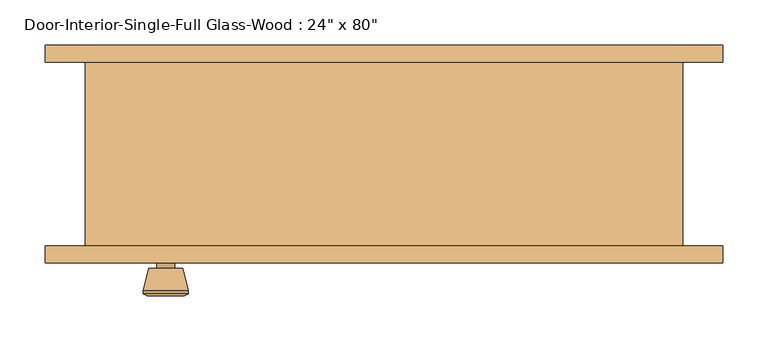
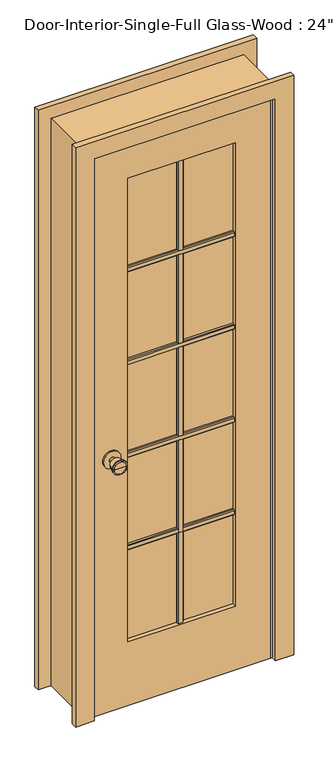
"""IFC4 building model written with IfcOpenShell, lengths in millimetres: door geometry."""

from ifc_helpers import new_model, si_unit, point, frame, frame_2d, origin, place, context, project, spatial, polyline, circle_curve, trimmed, segment, composite_curve, outline, extrude, faceted_brep, source, transform, mapped, element, save
from ifc_brep_helpers import plane_surface, cylinder_surface, revolved_surface, advanced_brep


def door_4bd6b2e0(model_context):
    return source(origin(), model_context, "Body", "SolidModel", [
        extrude(outline(polyline([(-84.455, 1586.23), (-84.455, 1567.18), (-90.805, 1567.18), (-93.98, 1570.355), (-93.98, 1583.055), (-90.805, 1586.23), (-84.455, 1586.23)])), frame((-184.15, 0.0, 0.0), z_axis=(1.0, 0.0, 0.0), x_axis=(0.0, 1.0, 0.0)), (0.0, 0.0, 1.0), 368.3),
        extrude(outline(polyline([(-84.455, 1249.9975), (-84.455, 1230.9475), (-90.805, 1230.9475), (-93.98, 1234.1225), (-93.98, 1246.8225), (-90.805, 1249.9975), (-84.455, 1249.9975)])), frame((-184.15, 0.0, 0.0), z_axis=(1.0, 0.0, 0.0), x_axis=(0.0, 1.0, 0.0)), (0.0, 0.0, 1.0), 368.3),
        extrude(outline(polyline([(-84.455, 913.765), (-84.455, 894.715), (-90.805, 894.715), (-93.98, 897.89), (-93.98, 910.59), (-90.805, 913.765), (-84.455, 913.765)])), frame((-184.15, 0.0, 0.0), z_axis=(1.0, 0.0, 0.0), x_axis=(0.0, 1.0, 0.0)), (0.0, 0.0, 1.0), 368.3),
        extrude(outline(polyline([(-9.525, -84.455), (9.525, -84.455), (9.525, -90.805), (6.35, -93.98), (-6.35, -93.98), (-9.525, -90.805), (-9.525, -84.455)])), frame((0.0, 0.0, 231.775), z_axis=(0.0, 0.0, 1.0), x_axis=(1.0, 0.0, 0.0)), (0.0, 0.0, 1.0), 1681.1625),
        extrude(outline(polyline([(-84.455, 577.5325), (-84.455, 558.4825), (-90.805, 558.4825), (-93.98, 561.6575), (-93.98, 574.3575), (-90.805, 577.5325), (-84.455, 577.5325)])), frame((-184.15, 0.0, 0.0), z_axis=(1.0, 0.0, 0.0), x_axis=(0.0, 1.0, 0.0)), (0.0, 0.0, 1.0), 368.3),
        extrude(outline(polyline([(-77.47, 1586.23), (-71.12, 1586.23), (-67.945, 1583.055), (-67.945, 1570.355), (-71.12, 1567.18), (-77.47, 1567.18), (-77.47, 1586.23)])), frame((-184.15, 0.0, 0.0), z_axis=(1.0, 0.0, 0.0), x_axis=(0.0, 1.0, 0.0)), (0.0, 0.0, 1.0), 368.3),
        extrude(outline(polyline([(-77.47, 1249.9975), (-71.12, 1249.9975), (-67.945, 1246.8225), (-67.945, 1234.1225), (-71.12, 1230.9475), (-77.47, 1230.9475), (-77.47, 1249.9975)])), frame((-184.15, 0.0, 0.0), z_axis=(1.0, 0.0, 0.0), x_axis=(0.0, 1.0, 0.0)), (0.0, 0.0, 1.0), 368.3),
        extrude(outline(polyline([(-77.47, 913.765), (-71.12, 913.765), (-67.945, 910.59), (-67.945, 897.89), (-71.12, 894.715), (-77.47, 894.715), (-77.47, 913.765)])), frame((-184.15, 0.0, 0.0), z_axis=(1.0, 0.0, 0.0), x_axis=(0.0, 1.0, 0.0)), (0.0, 0.0, 1.0), 368.3),
        extrude(outline(polyline([(-9.525, -77.47), (-9.525, -71.12), (-6.35, -67.945), (6.35, -67.945), (9.525, -71.12), (9.525, -77.47), (-9.525, -77.47)])), frame((0.0, 0.0, 231.775), z_axis=(0.0, 0.0, 1.0), x_axis=(1.0, 0.0, 0.0)), (0.0, 0.0, 1.0), 1681.1625),
        extrude(outline(polyline([(-77.47, 577.5325), (-71.12, 577.5325), (-67.945, 574.3575), (-67.945, 561.6575), (-71.12, 558.4825), (-77.47, 558.4825), (-77.47, 577.5325)])), frame((-184.15, 0.0, 0.0), z_axis=(1.0, 0.0, 0.0), x_axis=(0.0, 1.0, 0.0)), (0.0, 0.0, 1.0), 368.3),
        advanced_brep(
        [(-241.3, -57.5, 914.4), (-251.3, -57.5, 914.4), (-231.3, -57.5, 914.4), (-220.8241324, -8.5, 914.4), (-261.7758676, -8.5, 914.4), (-241.3, -8.5, 914.4), (-216.3, -10.3278681, 914.4), (-266.3, -10.3278681, 914.4), (-216.3, -13.7915463, 914.4), (-266.3, -13.7915463, 914.4), (-222.663764, -38.5, 914.4), (-259.936236, -38.5, 914.4), (-231.3, -38.5, 914.4), (-251.3, -38.5, 914.4)],
        [
            (0, 1),
            (1, 2, circle_curve(frame((-241.3, -57.5, 914.4), z_axis=(0.0, -1.0, 0.0), x_axis=(-1.0, 0.0, 0.0)), 10.0)),
            (2, 0),
            (2, 1, circle_curve(frame((-241.3, -57.5, 914.4), z_axis=(0.0, -1.0, 0.0), x_axis=(-1.0, 0.0, 0.0)), 10.0)),
            (3, 4, circle_curve(frame((-241.3, -8.5, 914.4), z_axis=(0.0, 1.0, 0.0), x_axis=(-1.0, 0.0, 0.0)), 20.4758676)),
            (4, 5),
            (5, 3),
            (4, 3, circle_curve(frame((-241.3, -8.5, 914.4), z_axis=(0.0, 1.0, 0.0), x_axis=(-1.0, 0.0, 0.0)), 20.4758676)),
            (6, 7, circle_curve(frame((-241.3, -10.3278681, 914.4), z_axis=(0.0, 1.0, 0.0), x_axis=(-1.0, 0.0, 0.0)), 25.0)),
            (7, 4),
            (3, 6),
            (7, 6, circle_curve(frame((-241.3, -10.3278681, 914.4), z_axis=(0.0, 1.0, 0.0), x_axis=(-1.0, 0.0, 0.0)), 25.0)),
            (8, 9, circle_curve(frame((-241.3, -13.7915463, 914.4), z_axis=(0.0, 1.0, 0.0), x_axis=(-1.0, 0.0, 0.0)), 25.0)),
            (9, 7),
            (6, 8),
            (9, 8, circle_curve(frame((-241.3, -13.7915463, 914.4), z_axis=(0.0, 1.0, 0.0), x_axis=(-1.0, 0.0, 0.0)), 25.0)),
            (10, 11, circle_curve(frame((-241.3, -38.5, 914.4), z_axis=(0.0, 1.0, 0.0), x_axis=(-1.0, 0.0, 0.0)), 18.636236)),
            (11, 9),
            (8, 10),
            (11, 10, circle_curve(frame((-241.3, -38.5, 914.4), z_axis=(0.0, 1.0, 0.0), x_axis=(-1.0, 0.0, 0.0)), 18.636236)),
            (12, 13, circle_curve(frame((-241.3, -38.5, 914.4), z_axis=(0.0, 1.0, 0.0), x_axis=(-1.0, 0.0, 0.0)), 10.0)),
            (13, 11),
            (10, 12),
            (13, 12, circle_curve(frame((-241.3, -38.5, 914.4), z_axis=(0.0, 1.0, 0.0), x_axis=(-1.0, 0.0, 0.0)), 10.0)),
            (1, 13),
            (12, 2),
        ],
        [
            plane_surface(frame((-241.3, -57.5, 914.4), z_axis=(0.0, -1.0, 0.0), x_axis=(-1.0, 0.0, 0.0))),
            plane_surface(frame((-241.3, -8.5, 914.4), z_axis=(0.0, 1.0, 0.0), x_axis=(-1.0, 0.0, 0.0))),
            revolved_surface(polyline([(-261.7758676, -8.5, 914.4), (-266.3, -10.3278681, 914.4)]), (-241.3, -57.5, 914.4), (0.0, -1.0, 0.0)),
            cylinder_surface(frame((-241.3, -57.5, 914.4), z_axis=(0.0, -1.0, 0.0), x_axis=(-1.0, 0.0, 0.0)), 25.0),
            revolved_surface(polyline([(-266.3, -13.7915463, 914.4), (-259.936236, -38.5, 914.4)]), (-241.3, -57.5, 914.4), (0.0, -1.0, 0.0)),
            plane_surface(frame((-241.3, -38.5, 914.4), z_axis=(0.0, -1.0, 0.0), x_axis=(-1.0, 0.0, 0.0))),
            cylinder_surface(frame((-241.3, -57.5, 914.4), z_axis=(0.0, -1.0, 0.0), x_axis=(-1.0, 0.0, 0.0)), 10.0),
        ],
        [
            (0, [[1, 2, 3]]),
            (0, [[-3, 4, -1]]),
            (1, [[5, 6, 7]]),
            (1, [[8, -7, -6]]),
            (2, [[9, 10, -5, 11]]),
            (2, [[12, -11, -8, -10]]),
            (3, [[13, 14, -9, 15]]),
            (3, [[16, -15, -12, -14]]),
            (4, [[17, 18, -13, 19]]),
            (4, [[20, -19, -16, -18]]),
            (5, [[21, 22, -17, 23]]),
            (5, [[24, -23, -20, -22]]),
            (6, [[-2, 25, -21, 26]]),
            (6, [[-4, -26, -24, -25]]),
        ],
    ),
        extrude(outline(composite_curve([segment(trimmed(circle_curve(frame_2d((914.4, -241.3)), 30.0), [point((914.4, -271.3))], [point((914.4, -211.3))], False, "CARTESIAN"), True, "CONTINUOUS"), segment(trimmed(circle_curve(frame_2d((914.4, -241.3)), 30.0), [point((914.4, -211.3))], [point((914.4, -271.3))], False, "CARTESIAN"), True, "CONTINUOUS")], self_intersect=False)), frame((0.0, -63.5, 0.0), z_axis=(0.0, 1.0, 0.0), x_axis=(0.0, 0.0, 1.0)), (0.0, 0.0, 1.0), 6.0),
        advanced_brep(
        [(-241.3, -104.425, 914.4), (-231.3, -104.425, 914.4), (-251.3, -104.425, 914.4), (-220.8241324, -153.425, 914.4), (-241.3, -153.425, 914.4), (-261.7758676, -153.425, 914.4), (-216.3, -151.5971319, 914.4), (-266.3, -151.5971319, 914.4), (-216.3, -148.1334537, 914.4), (-266.3, -148.1334537, 914.4), (-222.663764, -123.425, 914.4), (-259.936236, -123.425, 914.4), (-231.3, -123.425, 914.4), (-251.3, -123.425, 914.4)],
        [
            (0, 1),
            (1, 2, circle_curve(frame((-241.3, -104.425, 914.4), z_axis=(0.0, 1.0, 0.0), x_axis=(-1.0, 0.0, 0.0)), 10.0)),
            (2, 0),
            (2, 1, circle_curve(frame((-241.3, -104.425, 914.4), z_axis=(0.0, 1.0, 0.0), x_axis=(-1.0, 0.0, 0.0)), 10.0)),
            (3, 4),
            (4, 5),
            (5, 3, circle_curve(frame((-241.3, -153.425, 914.4), z_axis=(0.0, -1.0, 0.0), x_axis=(-1.0, 0.0, 0.0)), 20.4758676)),
            (3, 5, circle_curve(frame((-241.3, -153.425, 914.4), z_axis=(0.0, -1.0, 0.0), x_axis=(-1.0, 0.0, 0.0)), 20.4758676)),
            (6, 3),
            (5, 7),
            (7, 6, circle_curve(frame((-241.3, -151.5971319, 914.4), z_axis=(0.0, -1.0, 0.0), x_axis=(-1.0, 0.0, 0.0)), 25.0)),
            (6, 7, circle_curve(frame((-241.3, -151.5971319, 914.4), z_axis=(0.0, -1.0, 0.0), x_axis=(-1.0, 0.0, 0.0)), 25.0)),
            (8, 6),
            (7, 9),
            (9, 8, circle_curve(frame((-241.3, -148.1334537, 914.4), z_axis=(0.0, -1.0, 0.0), x_axis=(-1.0, 0.0, 0.0)), 25.0)),
            (8, 9, circle_curve(frame((-241.3, -148.1334537, 914.4), z_axis=(0.0, -1.0, 0.0), x_axis=(-1.0, 0.0, 0.0)), 25.0)),
            (10, 8),
            (9, 11),
            (11, 10, circle_curve(frame((-241.3, -123.425, 914.4), z_axis=(0.0, -1.0, 0.0), x_axis=(-1.0, 0.0, 0.0)), 18.636236)),
            (10, 11, circle_curve(frame((-241.3, -123.425, 914.4), z_axis=(0.0, -1.0, 0.0), x_axis=(-1.0, 0.0, 0.0)), 18.636236)),
            (12, 10),
            (11, 13),
            (13, 12, circle_curve(frame((-241.3, -123.425, 914.4), z_axis=(0.0, -1.0, 0.0), x_axis=(-1.0, 0.0, 0.0)), 10.0)),
            (12, 13, circle_curve(frame((-241.3, -123.425, 914.4), z_axis=(0.0, -1.0, 0.0), x_axis=(-1.0, 0.0, 0.0)), 10.0)),
            (1, 12),
            (13, 2),
        ],
        [
            plane_surface(frame((-241.3, -104.425, 914.4), z_axis=(0.0, 1.0, 0.0), x_axis=(-1.0, 0.0, 0.0))),
            plane_surface(frame((-241.3, -153.425, 914.4), z_axis=(0.0, -1.0, 0.0), x_axis=(-1.0, 0.0, 0.0))),
            revolved_surface(polyline([(-261.7758676, -153.425, 914.4), (-266.3, -151.5971319, 914.4)]), (-241.3, -104.425, 914.4), (0.0, 1.0, 0.0)),
            cylinder_surface(frame((-241.3, -104.425, 914.4), z_axis=(0.0, 1.0, 0.0), x_axis=(-1.0, 0.0, 0.0)), 25.0),
            revolved_surface(polyline([(-266.3, -148.1334537, 914.4), (-259.936236, -123.425, 914.4)]), (-241.3, -104.425, 914.4), (0.0, 1.0, 0.0)),
            plane_surface(frame((-241.3, -123.425, 914.4), z_axis=(0.0, 1.0, 0.0), x_axis=(-1.0, 0.0, 0.0))),
            cylinder_surface(frame((-241.3, -104.425, 914.4), z_axis=(0.0, 1.0, 0.0), x_axis=(-1.0, 0.0, 0.0)), 10.0),
        ],
        [
            (0, [[1, 2, 3]]),
            (0, [[-3, 4, -1]]),
            (1, [[5, 6, 7]]),
            (1, [[-6, -5, 8]]),
            (2, [[9, -7, 10, 11]]),
            (2, [[-10, -8, -9, 12]]),
            (3, [[13, -11, 14, 15]]),
            (3, [[-14, -12, -13, 16]]),
            (4, [[17, -15, 18, 19]]),
            (4, [[-18, -16, -17, 20]]),
            (5, [[21, -19, 22, 23]]),
            (5, [[-22, -20, -21, 24]]),
            (6, [[25, -23, 26, -2]]),
            (6, [[-26, -24, -25, -4]]),
        ],
    ),
        extrude(outline(composite_curve([segment(trimmed(circle_curve(frame_2d((914.4, -241.3)), 30.0), [point((914.4, -271.3))], [point((914.4, -211.3))], False, "CARTESIAN"), True, "CONTINUOUS"), segment(trimmed(circle_curve(frame_2d((914.4, -241.3)), 30.0), [point((914.4, -211.3))], [point((914.4, -271.3))], False, "CARTESIAN"), True, "CONTINUOUS")], self_intersect=False)), frame((0.0, -104.425, 0.0), z_axis=(0.0, 1.0, 0.0), x_axis=(0.0, 0.0, 1.0)), (0.0, 0.0, 1.0), 6.0),
        extrude(outline(polyline([(2032.0, -304.8), (0.0, -304.8), (0.0, 304.8), (2032.0, 304.8), (2032.0, -304.8)]), holes=[polyline([(1912.9375, -184.15), (1912.9375, 184.15), (231.775, 184.15), (231.775, -184.15), (1912.9375, -184.15)])]), frame((0.0, -98.425, 0.0), z_axis=(0.0, 1.0, 0.0), x_axis=(0.0, 0.0, 1.0)), (0.0, 0.0, 1.0), 34.925),
        faceted_brep([(330.2, -98.425, 0.0), (304.8, -98.425, 0.0), (304.8, -63.5, 0.0), (292.1, -63.5, 0.0), (292.1, -28.575, 0.0), (304.8, -28.575, 0.0), (304.8, 104.775, 0.0), (330.2, 104.775, 0.0), (330.2, 104.775, 2057.4), (330.2, -98.425, 2057.4), (304.8, 104.775, 2032.0), (-304.8, 104.775, 2032.0), (-304.8, 104.775, 0.0), (-330.2, 104.775, 0.0), (-330.2, 104.775, 2057.4), (304.8, -28.575, 2032.0), (292.1, -28.575, 2019.3), (-292.1, -28.575, 2019.3), (-292.1, -28.575, 0.0), (-304.8, -28.575, 0.0), (-304.8, -28.575, 2032.0), (292.1, -63.5, 2019.3), (304.8, -63.5, 2032.0), (-304.8, -63.5, 2032.0), (-304.8, -63.5, 0.0), (-292.1, -63.5, 0.0), (-292.1, -63.5, 2019.3), (304.8, -98.425, 2032.0), (-330.2, -98.425, 2057.4), (-330.2, -98.425, 0.0), (-304.8, -98.425, 0.0), (-304.8, -98.425, 2032.0)], [[[0, 1, 2, 3, 4, 5, 6, 7]], [[7, 8, 9, 0]], [[6, 10, 11, 12, 13, 14, 8, 7]], [[5, 15, 10, 6]], [[4, 16, 17, 18, 19, 20, 15, 5]], [[3, 21, 16, 4]], [[2, 22, 23, 24, 25, 26, 21, 3]], [[1, 27, 22, 2]], [[0, 9, 28, 29, 30, 31, 27, 1]], [[8, 14, 28, 9]], [[15, 20, 11, 10]], [[21, 26, 17, 16]], [[27, 31, 23, 22]], [[29, 13, 12, 19, 18, 25, 24, 30]], [[14, 13, 29, 28]], [[20, 19, 12, 11]], [[26, 25, 18, 17]], [[31, 30, 24, 23]]]),
        extrude(outline(polyline([(184.15, -77.47), (184.15, -84.455), (-184.15, -84.455), (-184.15, -77.47), (184.15, -77.47)])), frame((0.0, 0.0, 231.775), z_axis=(0.0, 0.0, 1.0), x_axis=(1.0, 0.0, 0.0)), (0.0, 0.0, 1.0), 1681.1625),
        extrude(outline(polyline([(0.0, 374.65), (2101.85, 374.65), (2101.85, -374.65), (0.0, -374.65), (0.0, -311.15), (2038.35, -311.15), (2038.35, 311.15), (0.0, 311.15), (0.0, 374.65)])), frame((0.0, 104.775, 0.0), z_axis=(0.0, 1.0, 0.0), x_axis=(0.0, 0.0, 1.0)), (0.0, 0.0, 1.0), 19.05),
        extrude(outline(polyline([(0.0, 374.65), (2101.85, 374.65), (2101.85, -374.65), (0.0, -374.65), (0.0, -311.15), (2038.35, -311.15), (2038.35, 311.15), (0.0, 311.15), (0.0, 374.65)])), frame((0.0, -117.475, 0.0), z_axis=(0.0, 1.0, 0.0), x_axis=(0.0, 0.0, 1.0)), (0.0, 0.0, 1.0), 19.05),
    ])


if __name__ == "__main__":
    model = new_model("IFC4")
    model_context = context("Model", 3, world=origin())
    ifc_project = project(units=[si_unit("LENGTHUNIT", "METRE", prefix="MILLI")], contexts=[model_context])
    site = spatial("IfcSite", under=ifc_project)
    building = spatial("IfcBuilding", under=site)
    placement = place(None, origin())
    door_shape = door_4bd6b2e0(model_context)
    element("IfcDoor", 1, ObjectType="Door-Interior-Single-Full Glass-Wood : 24\" x 80\"", at=placement, inside=building, context=model_context, shape_type="MappedRepresentation", body=[
        mapped(door_shape, transform((0.0, 0.0, 0.0), x_axis=(1.0, 0.0, 0.0), y_axis=(0.0, 1.0, 0.0), z_axis=(0.0, 0.0, 1.0))),
    ])
    save(model, "model.ifc")

# Revit data of these elements
# Type "Door-Interior-Single-Full Glass-Wood : 24\" x 80\""
#   Type Mark = "10"
#   Assembly Code = "C1020300"
#   Analytic Construction = "Wood frame with single clear glass"
#   Top Rail = 0' - 4 11/16"
#   Thickness = 0' - 1 3/8"
#   Thermal Resistance (R) = 1.0102 (h·ft²·°F)/BTU
#   Swing Angle [instance default] = 90.00°
#   Stiles = 0' - 4 3/4"
#   Rough Width = 2' - 2"
#   Rough Height = 6' - 9"
#   Height = 6' - 8"
#   Width = 2' - 0"
#   Heat Transfer Coefficient (U) = 0.9900 BTU/(h·ft²·°F)
#   Bottom Rail = 0' - 9 1/8"
#   Show Grill [instance default] = yes
#   Trim Material = Cherry
#   Panel Material = Cherry
#   Frame Material = Cherry
#   Door Handle Material = Aluminum
#   Visual Light Transmittance = 0
#   Solar Heat Gain Coefficient = 0
#   Wall Closure = (empty or 0)
#   Function = (empty or 0)
# Element 1 (IfcDoor, "Door-Interior-Single-Full Glass-Wood : 24\" x 80\"")
#   Materials on its faces: "Cherry", "Aluminum", "Glass"
# Materials
#   "Cherry": class "Wood", colour RGB 226 177 128, transparency 0, Description = "Prunus Serotina", Cost = 0
#   "Aluminum": class "Metal", colour RGB 247 247 247, transparency 0, Description = "Aluminum 6061", Cost = 0
#   "Glass": class "Glass", colour RGB 0 128 192, transparency 0.75, Description = "Soda Lime Glass", Cost = 0
